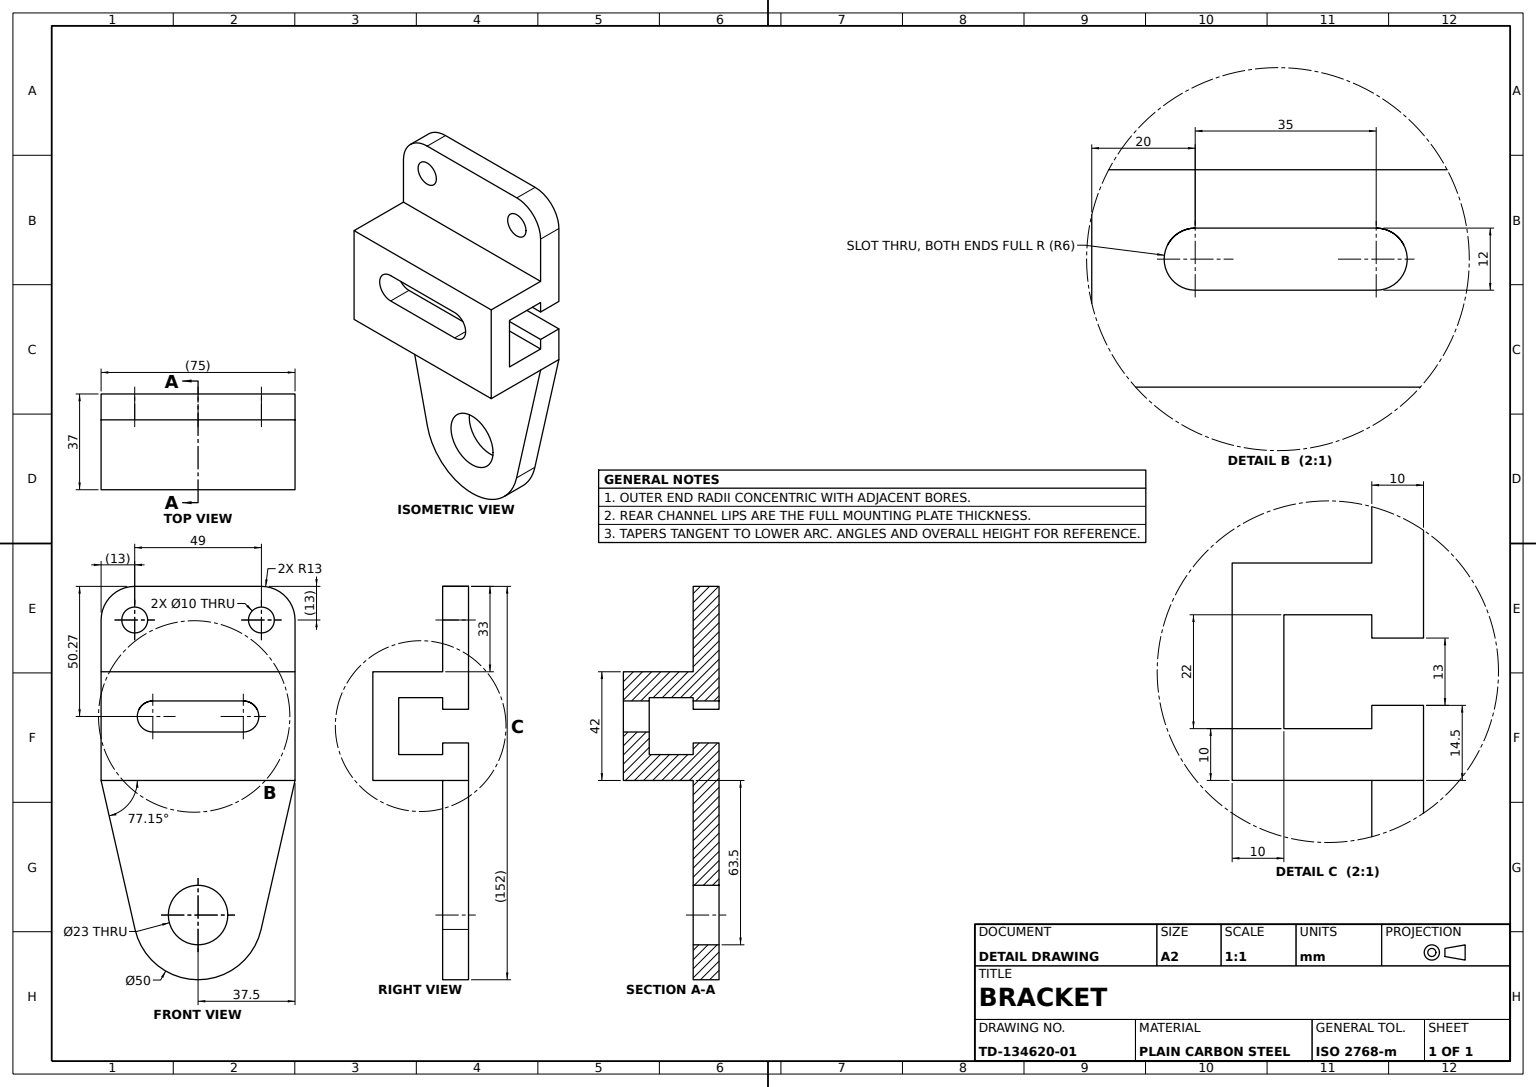
from build123d import *

# Parameters (mm, degrees)
BRACKET_PROFILE_SKETCH_R        = 5
BRACKET_PROFILE_SKETCH_R_2      = 11.5
BRACKET_BODY_DEPTH              = 37
SLOT_AND_CHANNEL_CUT_DEPTH      = 103.992718189
SLOT_AND_CHANNEL_CUT_DEPTH_BACK = 103.992718189
SLOT_AND_CHANNEL_SKETCH_W       = 27
SLOT_AND_CHANNEL_SKETCH_H       = 33
SLOT_AND_CHANNEL_SKETCH_H_2     = 77


with BuildPart() as part:
    # Bracket Profile Sketch → Bracket Body (new body)
    with BuildSketch(Plane.XY):
        with BuildLine():
            Line((-24.5, 63.5), (24.5, 63.5))
            ThreePointArc((24.5, 63.5), (33.692388155, 59.692388155), (37.5, 50.5))
            Line((37.5, 50.5), (37.5, -11.5))
            Line((37.5, -11.5), (24.374261359, -69.058361557))
            ThreePointArc((24.374261359, -69.058361557), (0, -88.5), (-24.374261359, -69.058361557))
            Line((-24.374261359, -69.058361557), (-37.5, -11.5))
            Line((-37.5, -11.5), (-37.5, 50.5))
            ThreePointArc((-37.5, 50.5), (-33.692388155, 59.692388155), (-24.5, 63.5))
        make_face()
        with Locations((24.5, 50.5)):
            Circle(BRACKET_PROFILE_SKETCH_R, mode=Mode.SUBTRACT)
        with Locations((-24.5, 50.5)):
            Circle(BRACKET_PROFILE_SKETCH_R, mode=Mode.SUBTRACT)
        with Locations((0, -63.5)):
            Circle(BRACKET_PROFILE_SKETCH_R_2, mode=Mode.SUBTRACT)
        with BuildLine():
            ThreePointArc((17.5, 7.226797096), (23.5, 13.226797096), (17.5, 19.226797096))
            Line((17.5, 19.226797096), (-17.5, 19.226797096))
            ThreePointArc((-17.5, 19.226797096), (-23.5, 13.226797096), (-17.5, 7.226797096))
            Line((-17.5, 7.226797096), (17.5, 7.226797096))
        make_face(mode=Mode.SUBTRACT)
    extrude(amount=BRACKET_BODY_DEPTH)

    # Slot and Channel Sketch → Slot and Channel Cut (cut, two sides: drawn at the far end of the back side and taken through both)
    with BuildSketch(Plane(origin=(0, 0, 0), x_dir=(0, 0, -1), z_dir=(1, 0, 0)).offset(-SLOT_AND_CHANNEL_CUT_DEPTH_BACK)):
        with Locations((-23.5, 47)):
            Rectangle(SLOT_AND_CHANNEL_SKETCH_W, SLOT_AND_CHANNEL_SKETCH_H)
        Polygon((0, 3), (0, 16), (-10, 16), (-10, 20.5), (-27, 20.5), (-27, -1.5), (-10, -1.5), (-10, 3), align=None)
        with Locations((-23.5, -50)):
            Rectangle(SLOT_AND_CHANNEL_SKETCH_W, SLOT_AND_CHANNEL_SKETCH_H_2)
    extrude(amount=SLOT_AND_CHANNEL_CUT_DEPTH + SLOT_AND_CHANNEL_CUT_DEPTH_BACK, mode=Mode.SUBTRACT)


solid = part.part
